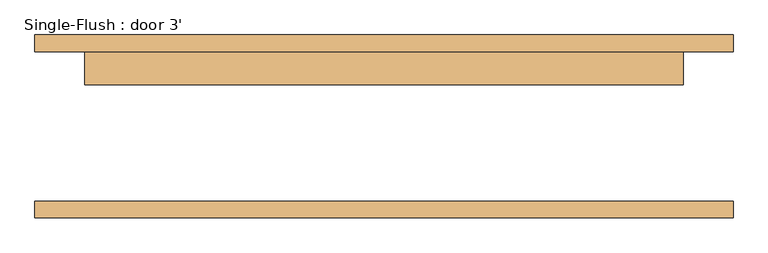
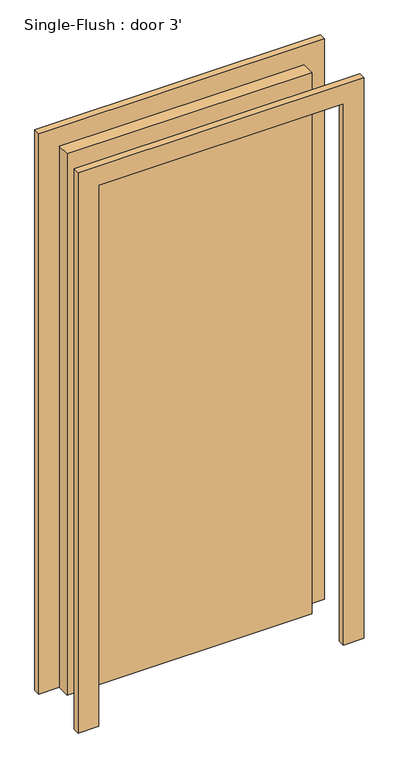
"""IFC4 building model written with IfcOpenShell, lengths in millimetres: door geometry, Single-Flush : door 3'."""

from ifc_helpers import new_model, si_unit, frame, origin, origin_with_axes, place, context, project, spatial, polyline, outline, extrude, source, transform, mapped, element, save


def single_flush_door_3_0ca8825f(model_context):
    return source(origin(), model_context, "Body", "SweptSolid", [
        extrude(outline(polyline([(2209.8, -533.4), (0.0, -533.4), (0.0, -457.2), (2133.6, -457.2), (2133.6, 457.2), (0.0, 457.2), (0.0, 533.4), (2209.8, 533.4), (2209.8, -533.4)])), frame((0.0, 114.3, 0.0), z_axis=(0.0, 1.0, 0.0), x_axis=(0.0, 0.0, 1.0)), (0.0, 0.0, 1.0), 25.4),
        extrude(outline(polyline([(2209.8, 533.4), (2209.8, -533.4), (0.0, -533.4), (0.0, -457.2), (2133.6, -457.2), (2133.6, 457.2), (0.0, 457.2), (0.0, 533.4), (2209.8, 533.4)])), frame((0.0, -139.7, 0.0), z_axis=(0.0, 1.0, 0.0), x_axis=(0.0, 0.0, 1.0)), (0.0, 0.0, 1.0), 25.4),
        extrude(outline(polyline([(457.2, 63.5), (-457.2, 63.5), (-457.2, 114.3), (457.2, 114.3), (457.2, 63.5)])), origin_with_axes(), (0.0, 0.0, 1.0), 2133.6),
    ])


if __name__ == "__main__":
    model = new_model("IFC4")
    model_context = context("Model", 3, world=origin())
    ifc_project = project(units=[si_unit("LENGTHUNIT", "METRE", prefix="MILLI")], contexts=[model_context])
    site = spatial("IfcSite", under=ifc_project)
    building = spatial("IfcBuilding", under=site)
    placement = place(None, origin())
    single_flush_door_3_shape = single_flush_door_3_0ca8825f(model_context)
    element("IfcDoor", 1, ObjectType="Single-Flush : door 3'", at=placement, inside=building, context=model_context, shape_type="MappedRepresentation", body=[
        mapped(single_flush_door_3_shape, transform((0.0, 0.0, 0.0), x_axis=(1.0, 0.0, 0.0), y_axis=(0.0, 1.0, 0.0), z_axis=(0.0, 0.0, 1.0))),
    ])
    save(model, "model.ifc")

# Revit data of these elements
# Type "Single-Flush : door 3'"
#   Type Mark = "8"
#   Construction Type Id = "MDOOR"
#   Assembly Code = "C1020"
#   Analytic Construction = "Metal"
#   Thickness = 0' - 2"
#   Heat Transfer Coefficient (U) = 0.651978 BTU/(h·ft²·°F)
#   Height = 7' - 0"
#   Trim Projection Ext = 0' - 1"
#   Trim Projection Int = 0' - 1"
#   Trim Width = 0' - 3"
#   Width = 3' - 0"
#   Define Thermal Properties by = 1
#   Door Material = Door - Panel
#   Frame Material = Door - Frame
#   Visual Light Transmittance = 0
#   Solar Heat Gain Coefficient = 0
#   Function = (empty or 0)
#   Wall Closure = (empty or 0)
# Element 1 (IfcDoor, "Single-Flush : door 3'")
#   Materials on its faces: "Door - Frame", "Door - Panel"
# Materials
#   "Door - Panel": class "Wood", colour RGB 210 159 95, transparency 0, Cost = 0
#   "Door - Frame": colour RGB 118 70 51, transparency 0, Cost = 0
